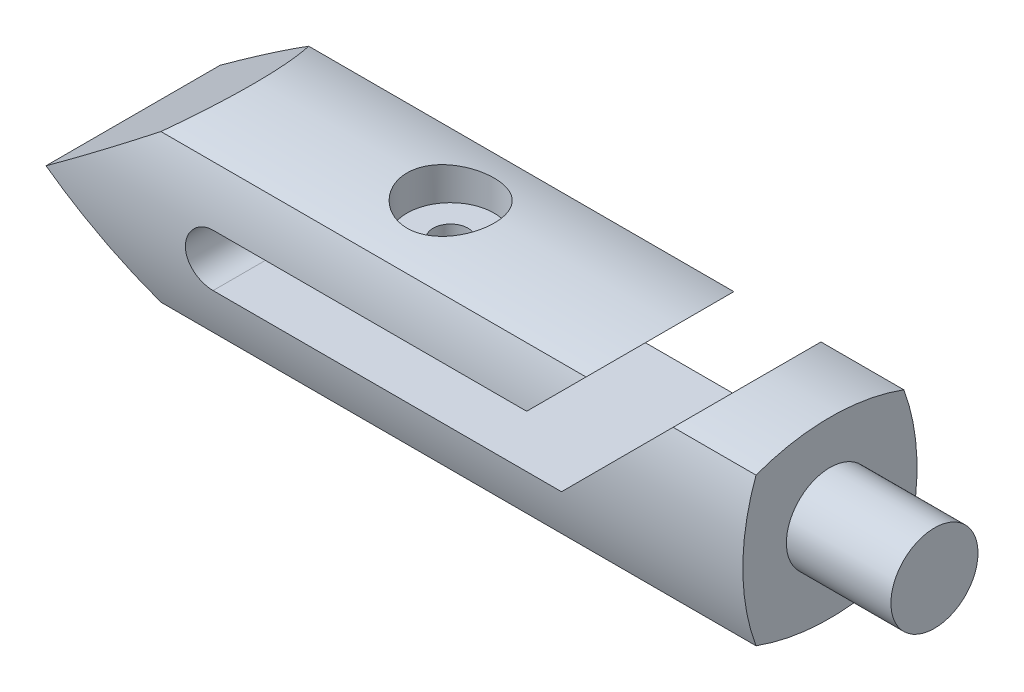
ISO-10303-21;
HEADER;
FILE_DESCRIPTION(('STEP AP214'),'2;1');
FILE_NAME('part.step','',(''),(''),'','','');
FILE_SCHEMA(('AUTOMOTIVE_DESIGN { 1 0 10303 214 1 1 1 1 }'));
ENDSEC;
DATA;
#1=APPLICATION_CONTEXT('core data for automotive mechanical design processes');
#2=APPLICATION_PROTOCOL_DEFINITION('international standard','automotive_design',2000,#1);
#3=PRODUCT_CONTEXT('',#1,'mechanical');
#4=PRODUCT('Part','Part','',(#3));
#5=PRODUCT_RELATED_PRODUCT_CATEGORY('part','',(#4));
#6=PRODUCT_DEFINITION_FORMATION('','',#4);
#7=PRODUCT_DEFINITION_CONTEXT('part definition',#1,'design');
#8=PRODUCT_DEFINITION('design','',#6,#7);
#9=PRODUCT_DEFINITION_SHAPE('','',#8);
#10=(LENGTH_UNIT() NAMED_UNIT(*) SI_UNIT(.MILLI.,.METRE.));
#11=(NAMED_UNIT(*) PLANE_ANGLE_UNIT() SI_UNIT($,.RADIAN.));
#12=(NAMED_UNIT(*) SI_UNIT($,.STERADIAN.) SOLID_ANGLE_UNIT());
#13=UNCERTAINTY_MEASURE_WITH_UNIT(LENGTH_MEASURE(1.E-05),#10,'distance_accuracy_value','');
#14=(GEOMETRIC_REPRESENTATION_CONTEXT(3) GLOBAL_UNCERTAINTY_ASSIGNED_CONTEXT((#13)) GLOBAL_UNIT_ASSIGNED_CONTEXT((#10,
#11,#12)) REPRESENTATION_CONTEXT('',''));
#15=CARTESIAN_POINT('',(0.,0.,0.));
#16=DIRECTION('',(0.,0.,1.));
#17=DIRECTION('',(1.,0.,0.));
#18=AXIS2_PLACEMENT_3D('',#15,#16,#17);
#19=CARTESIAN_POINT('',(80.,-14.5241496511874,0.));
#20=DIRECTION('',(-1.,0.,0.));
#21=DIRECTION('',(0.,0.,1.));
#22=AXIS2_PLACEMENT_3D('',#19,#20,#21);
#23=CYLINDRICAL_SURFACE('',#22,24.5241496511874);
#24=DIRECTION('',(-1.,0.,0.));
#25=VECTOR('',#24,1.);
#26=CARTESIAN_POINT('',(80.,8.48528137423857,-8.48528137423857));
#27=LINE('',#26,#25);
#28=CARTESIAN_POINT('',(80.,8.48528137423857,-8.48528137423857));
#29=VERTEX_POINT('',#28);
#30=CARTESIAN_POINT('',(70.4852813742386,8.48528137423857,-8.48528137423857));
#31=VERTEX_POINT('',#30);
#32=EDGE_CURVE('E248',#29,#31,#27,.T.);
#33=ORIENTED_EDGE('',*,*,#32,.T.);
#34=CARTESIAN_POINT('',(47.4758503488127,-14.5241496511874,0.));
#35=DIRECTION('',(0.707106781186549,-0.707106781186546,0.));
#36=DIRECTION('',(-0.707106781186546,-0.707106781186549,0.));
#37=AXIS2_PLACEMENT_3D('',#34,#35,#36);
#38=ELLIPSE('',#37,34.6823850423765,24.5241496511874);
#39=CARTESIAN_POINT('',(70.4852813742386,8.48528137423856,8.48528137423857));
#40=VERTEX_POINT('',#39);
#41=EDGE_CURVE('E190',#31,#40,#38,.T.);
#42=ORIENTED_EDGE('',*,*,#41,.T.);
#43=DIRECTION('',(-1.,0.,0.));
#44=VECTOR('',#43,1.);
#45=CARTESIAN_POINT('',(80.,8.48528137423856,8.48528137423857));
#46=LINE('',#45,#44);
#47=CARTESIAN_POINT('',(80.,8.48528137423856,8.48528137423857));
#48=VERTEX_POINT('',#47);
#49=EDGE_CURVE('E259',#48,#40,#46,.T.);
#50=ORIENTED_EDGE('',*,*,#49,.F.);
#51=CARTESIAN_POINT('',(80.,-14.5241496511874,0.));
#52=DIRECTION('',(1.,0.,0.));
#53=DIRECTION('',(0.,0.,1.));
#54=AXIS2_PLACEMENT_3D('',#51,#52,#53);
#55=CIRCLE('',#54,24.5241496511874);
#56=EDGE_CURVE('E251',#29,#48,#55,.T.);
#57=ORIENTED_EDGE('',*,*,#56,.F.);
#58=EDGE_LOOP('',(#33,#42,#50,#57));
#59=FACE_BOUND('',#58,.T.);
#60=ADVANCED_FACE('F37',(#59),#23,.T.);
#61=CARTESIAN_POINT('',(80.,14.5241496511874,0.));
#62=DIRECTION('',(-1.,0.,0.));
#63=DIRECTION('',(0.,0.,1.));
#64=AXIS2_PLACEMENT_3D('',#61,#62,#63);
#65=CYLINDRICAL_SURFACE('',#64,24.5241496511874);
#66=CARTESIAN_POINT('',(36.4274618149669,-9.91878279756692,1.99423404330306));
#67=CARTESIAN_POINT('',(36.5396107174262,-9.91878387951594,1.99422914378513));
#68=CARTESIAN_POINT('',(36.6518361731554,-9.91956063360397,1.98477026677701));
#69=CARTESIAN_POINT('',(36.8731828140898,-9.9225835690341,1.94717561648094));
#70=CARTESIAN_POINT('',(36.9823003258081,-9.92483141960828,1.91901862617786));
#71=CARTESIAN_POINT('',(37.1941934107136,-9.93053976466019,1.84484606293275));
#72=CARTESIAN_POINT('',(37.2969724958837,-9.93399958038463,1.79884048443032));
#73=CARTESIAN_POINT('',(37.4933243792085,-9.94174027856262,1.69029359217857));
#74=CARTESIAN_POINT('',(37.5868991571246,-9.94602098386358,1.62775584506402));
#75=CARTESIAN_POINT('',(37.7624342025995,-9.9549314009157,1.48775754496128));
#76=CARTESIAN_POINT('',(37.8443694897502,-9.95956183158808,1.41026571347757));
#77=CARTESIAN_POINT('',(37.9940848321214,-9.96864179702908,1.24262424200629));
#78=CARTESIAN_POINT('',(38.0618642803249,-9.97309132403378,1.15247405949275));
#79=CARTESIAN_POINT('',(38.181422340064,-9.98131288649792,0.961931970770378));
#80=CARTESIAN_POINT('',(38.2331803569177,-9.98508404736901,0.861527101272117));
#81=CARTESIAN_POINT('',(38.3190935872972,-9.99151452425883,0.65341609960103));
#82=CARTESIAN_POINT('',(38.3532491009652,-9.99417385923528,0.545710091956111));
#83=CARTESIAN_POINT('',(38.4029140361771,-9.99807374981551,0.32631236962031));
#84=CARTESIAN_POINT('',(38.4184653849531,-9.99931749535021,0.214630203439155));
#85=CARTESIAN_POINT('',(38.4306113494179,-10.0002546641417,-0.00976557573688327));
#86=CARTESIAN_POINT('',(38.4272062949528,-9.99994811437399,-0.122479170750583));
#87=CARTESIAN_POINT('',(38.4015701990306,-9.99781961597193,-0.34546647047582));
#88=CARTESIAN_POINT('',(38.3793822976169,-9.99600114006806,-0.455745172544806));
#89=CARTESIAN_POINT('',(38.3168786032461,-9.99105507660593,-0.67100838413095));
#90=CARTESIAN_POINT('',(38.2765626316985,-9.98792747615073,-0.775992841479997));
#91=CARTESIAN_POINT('',(38.1788921277876,-9.98070629614845,-0.977841944245001));
#92=CARTESIAN_POINT('',(38.1215156897114,-9.9766114760856,-1.07469594383791));
#93=CARTESIAN_POINT('',(37.9913689733101,-9.96791439848711,-1.25741589796487));
#94=CARTESIAN_POINT('',(37.9185983918504,-9.9633121309599,-1.3432816360696));
#95=CARTESIAN_POINT('',(37.7594737792699,-9.95409985360554,-1.50185153497478));
#96=CARTESIAN_POINT('',(37.6730804520599,-9.94948986078113,-1.57451626919999));
#97=CARTESIAN_POINT('',(37.4892995271567,-9.94079402053666,-1.70431590707003));
#98=CARTESIAN_POINT('',(37.3919119255137,-9.9367081733049,-1.76145080513547));
#99=CARTESIAN_POINT('',(37.1888877575802,-9.92952175902326,-1.85856220639398));
#100=CARTESIAN_POINT('',(37.0832508828721,-9.92642122883369,-1.89853806769411));
#101=CARTESIAN_POINT('',(36.8667332709295,-9.92155756185618,-1.96017326130295));
#102=CARTESIAN_POINT('',(36.7558526431209,-9.91979439717337,-1.98183297565238));
#103=CARTESIAN_POINT('',(36.5323500030333,-9.91780917693866,-2.00616958067166));
#104=CARTESIAN_POINT('',(36.4197341898689,-9.91758252853865,-2.00890304490123));
#105=CARTESIAN_POINT('',(36.1956459444873,-9.91868382758372,-1.99545768529034));
#106=CARTESIAN_POINT('',(36.0841735016966,-9.92001176063949,-1.97927903650156));
#107=CARTESIAN_POINT('',(35.8656968809238,-9.92406876703792,-1.92851561407786));
#108=CARTESIAN_POINT('',(35.7586865961699,-9.92679585261481,-1.8939569502517));
#109=CARTESIAN_POINT('',(35.551982876258,-9.93334291111696,-1.80744148884544));
#110=CARTESIAN_POINT('',(35.4522895561389,-9.93716290122049,-1.75548441779515));
#111=CARTESIAN_POINT('',(35.26279284038,-9.94547740571136,-1.63550560894451));
#112=CARTESIAN_POINT('',(35.1730131914628,-9.94997348127245,-1.56744647508123));
#113=CARTESIAN_POINT('',(35.0061319756589,-9.959129613978,-1.41725031708977));
#114=CARTESIAN_POINT('',(34.9290306267771,-9.96378967394052,-1.33511305093606));
#115=CARTESIAN_POINT('',(34.7894999262584,-9.97276407920029,-1.15884676404799));
#116=CARTESIAN_POINT('',(34.7271076192201,-9.97707753395946,-1.06468836749474));
#117=CARTESIAN_POINT('',(34.6190195674161,-9.9848616206904,-0.867199529201713));
#118=CARTESIAN_POINT('',(34.5733236688444,-9.98833226042602,-0.763869171964319));
#119=CARTESIAN_POINT('',(34.4999846709961,-9.99403787574732,-0.551090485409505));
#120=CARTESIAN_POINT('',(34.4723205998467,-9.99627428633419,-0.441649424615883));
#121=CARTESIAN_POINT('',(34.4357636338553,-9.99926739888673,-0.219656585902366));
#122=CARTESIAN_POINT('',(34.426870394789,-10.0000241279872,-0.10710486506488));
#123=CARTESIAN_POINT('',(34.4281125479617,-9.99997475904181,0.117558752308689));
#124=CARTESIAN_POINT('',(34.4381917133107,-9.99917327869674,0.229670964829407));
#125=CARTESIAN_POINT('',(34.4769765751515,-9.99610895300196,0.450604543013426));
#126=CARTESIAN_POINT('',(34.5056822851811,-9.99384610659015,0.559425906284876));
#127=CARTESIAN_POINT('',(34.5808878132343,-9.98811548672665,0.770679710877488));
#128=CARTESIAN_POINT('',(34.6273847023371,-9.98464791161532,0.873113200593169));
#129=CARTESIAN_POINT('',(34.7368466796898,-9.97689787677331,1.0687283584638));
#130=CARTESIAN_POINT('',(34.7998114837321,-9.97261543110623,1.16191018624808));
#131=CARTESIAN_POINT('',(34.9406238598056,-9.96370373201027,1.3366530766732));
#132=CARTESIAN_POINT('',(35.0185112405738,-9.95907357154377,1.41818201368821));
#133=CARTESIAN_POINT('',(35.1868874368628,-9.94999734378366,1.56704257270282));
#134=CARTESIAN_POINT('',(35.277379304508,-9.94555132141762,1.63437074608838));
#135=CARTESIAN_POINT('',(35.4685683054161,-9.93733902638497,1.75300935209794));
#136=CARTESIAN_POINT('',(35.5692840696393,-9.93357403076966,1.8042898210522));
#137=CARTESIAN_POINT('',(35.7778571652447,-9.92716649272995,1.8891486623785));
#138=CARTESIAN_POINT('',(35.8857061163373,-9.92452265928407,1.92274740611571));
#139=CARTESIAN_POINT('',(36.0664045825854,-9.92133837222752,1.96271812167535));
#140=CARTESIAN_POINT('',(36.1380918860322,-9.92038443324707,1.97452093798435));
#141=CARTESIAN_POINT('',(36.2823293776411,-9.9191062965746,1.99028047462704));
#142=CARTESIAN_POINT('',(36.3548795636816,-9.91878209733451,1.99423721424842));
#143=CARTESIAN_POINT('',(36.4274618149669,-9.91878279756692,1.99423404330306));
#144=B_SPLINE_CURVE_WITH_KNOTS('',3,(#66,#67,#68,#69,#70,#71,#72,#73,#74,#75,#76,#77,#78,#79,
#80,#81,#82,#83,#84,#85,#86,#87,#88,#89,#90,#91,#92,#93,#94,#95,#96,#97,#98,#99,#100,#101,#102,
#103,#104,#105,#106,#107,#108,#109,#110,#111,#112,#113,#114,#115,#116,#117,#118,#119,#120,#121,
#122,#123,#124,#125,#126,#127,#128,#129,#130,#131,#132,#133,#134,#135,#136,#137,#138,#139,#140,
#141,#142,#143),.UNSPECIFIED.,.T.,.F.,(4,2,2,2,2,2,2,2,2,2,2,2,2,2,2,2,2,2,2,2,2,2,2,2,2,2,2,2,
2,2,2,2,2,2,2,2,2,2,4),(0.,0.336181721876391,0.672745567258664,1.00912122278101,
1.34542436807037,1.68243871436159,2.01946750920759,2.35692775427698,2.69438224508603,
3.03107479102768,3.36776147845564,3.70367696258342,4.03959575608857,4.37594774715791,
4.71230636213535,5.0496536092943,5.38700097765134,5.72436096455003,6.06171391457386,
6.39805802616283,6.73439902455492,7.07026350349091,7.40613326183175,7.74279084986612,
8.07945422616162,8.41695663863483,8.75445594198052,9.09156201385299,9.42866190373632,
9.76476433216564,10.1008670048747,10.4369143695644,10.7729559350427,11.109906760192,
11.4469393188911,11.784597468342,12.1218657406696,12.3394415319915,12.5570167884555),.UNSPECIFIED.);
#145=CARTESIAN_POINT('',(36.4274618149669,-9.91878279756692,1.99423404330306));
#146=VERTEX_POINT('',#145);
#147=EDGE_CURVE('E44',#146,#146,#144,.T.);
#148=ORIENTED_EDGE('',*,*,#147,.T.);
#149=EDGE_LOOP('',(#148));
#150=FACE_BOUND('',#149,.T.);
#151=CARTESIAN_POINT('',(-19.9907769901119,14.5241496511874,0.));
#152=DIRECTION('',(-0.587785252292474,-0.809016994374947,0.));
#153=DIRECTION('',(-0.809016994374947,0.587785252292474,0.));
#154=AXIS2_PLACEMENT_3D('',#151,#152,#153);
#155=ELLIPSE('',#154,41.7229754498578,24.5241496511874);
#156=CARTESIAN_POINT('',(11.6789878736127,-8.48528137423857,-8.48528137423857));
#157=VERTEX_POINT('',#156);
#158=CARTESIAN_POINT('',(11.6789878736127,-8.48528137423857,8.48528137423857));
#159=VERTEX_POINT('',#158);
#160=EDGE_CURVE('E289',#157,#159,#155,.T.);
#161=ORIENTED_EDGE('',*,*,#160,.F.);
#162=DIRECTION('',(-1.,0.,0.));
#163=VECTOR('',#162,1.);
#164=CARTESIAN_POINT('',(80.,-8.48528137423857,-8.48528137423857));
#165=LINE('',#164,#163);
#166=CARTESIAN_POINT('',(80.,-8.48528137423857,-8.48528137423857));
#167=VERTEX_POINT('',#166);
#168=EDGE_CURVE('E255',#167,#157,#165,.T.);
#169=ORIENTED_EDGE('',*,*,#168,.F.);
#170=CARTESIAN_POINT('',(80.,14.5241496511874,0.));
#171=DIRECTION('',(1.,0.,0.));
#172=DIRECTION('',(0.,0.,-1.));
#173=AXIS2_PLACEMENT_3D('',#170,#171,#172);
#174=CIRCLE('',#173,24.5241496511874);
#175=CARTESIAN_POINT('',(80.,-8.48528137423857,8.48528137423857));
#176=VERTEX_POINT('',#175);
#177=EDGE_CURVE('E303',#176,#167,#174,.T.);
#178=ORIENTED_EDGE('',*,*,#177,.F.);
#179=DIRECTION('',(-1.,0.,0.));
#180=VECTOR('',#179,1.);
#181=CARTESIAN_POINT('',(80.,-8.48528137423857,8.48528137423857));
#182=LINE('',#181,#180);
#183=EDGE_CURVE('E310',#176,#159,#182,.T.);
#184=ORIENTED_EDGE('',*,*,#183,.T.);
#185=EDGE_LOOP('',(#161,#169,#178,#184));
#186=FACE_BOUND('',#185,.T.);
#187=ADVANCED_FACE('F45',(#150,#186),#65,.T.);
#188=CARTESIAN_POINT('',(80.,0.,14.5241496511873));
#189=DIRECTION('',(-1.,0.,0.));
#190=DIRECTION('',(0.,0.,1.));
#191=AXIS2_PLACEMENT_3D('',#188,#189,#190);
#192=CYLINDRICAL_SURFACE('',#191,24.5241496511874);
#193=DIRECTION('',(-1.,0.,0.));
#194=VECTOR('',#193,1.);
#195=CARTESIAN_POINT('',(80.,3.,-9.81581575786434));
#196=LINE('',#195,#194);
#197=CARTESIAN_POINT('',(55.,3.,-9.81581575786434));
#198=VERTEX_POINT('',#197);
#199=CARTESIAN_POINT('',(19.,3.,-9.81581575786434));
#200=VERTEX_POINT('',#199);
#201=EDGE_CURVE('E134',#198,#200,#196,.T.);
#202=ORIENTED_EDGE('',*,*,#201,.T.);
#203=CARTESIAN_POINT('',(19.,3.,-9.81581575786434));
#204=CARTESIAN_POINT('',(18.9159581160124,3.00000845084196,-9.81581145497862));
#205=CARTESIAN_POINT('',(18.8319204963024,2.99646853759129,-9.81625094060136));
#206=CARTESIAN_POINT('',(18.664452727367,2.98235744015164,-9.81798568516386));
#207=CARTESIAN_POINT('',(18.5810225326003,2.97178678869135,-9.81928087926537));
#208=CARTESIAN_POINT('',(18.4154392675195,2.94369384169545,-9.82269352253626));
#209=CARTESIAN_POINT('',(18.3332849928944,2.92617857509987,-9.82481014026211));
#210=CARTESIAN_POINT('',(18.1707754863183,2.88434334207964,-9.82980114295365));
#211=CARTESIAN_POINT('',(18.0904202431902,2.86002341794395,-9.83267552321006));
#212=CARTESIAN_POINT('',(17.8528488125263,2.77707037687542,-9.8423220854026));
#213=CARTESIAN_POINT('',(17.6990342186838,2.7084281645373,-9.85011973385544));
#214=CARTESIAN_POINT('',(17.405204709813,2.54652833477299,-9.86756395041019));
#215=CARTESIAN_POINT('',(17.2651886506251,2.45327276062299,-9.87721036501874));
#216=CARTESIAN_POINT('',(17.0020707993755,2.24424237310175,-9.8973232696192));
#217=CARTESIAN_POINT('',(16.879051473348,2.1283639265146,-9.90779339591513));
#218=CARTESIAN_POINT('',(16.6541477560292,1.87759299766197,-9.9283421820244));
#219=CARTESIAN_POINT('',(16.5522665856149,1.74269762298811,-9.93842078198995));
#220=CARTESIAN_POINT('',(16.3722404196189,1.45720411210512,-9.95708742327201));
#221=CARTESIAN_POINT('',(16.2941710108273,1.30655796834562,-9.96567068163192));
#222=CARTESIAN_POINT('',(16.1644749648453,0.994180082275956,-9.98033855169631));
#223=CARTESIAN_POINT('',(16.1128458186752,0.832449393456734,-9.98642340046998));
#224=CARTESIAN_POINT('',(16.0377389031857,0.50334311382209,-9.99538359571057));
#225=CARTESIAN_POINT('',(16.0141216504363,0.335999795323433,-9.99827483953598));
#226=CARTESIAN_POINT('',(15.9952767735246,-0.00030237620532862,-10.000576353286));
#227=CARTESIAN_POINT('',(16.0000487651077,-0.169261207338216,-9.99998667032566));
#228=CARTESIAN_POINT('',(16.0377359374063,-0.503040463753467,-9.99540552373128));
#229=CARTESIAN_POINT('',(16.0705003118933,-0.667878202042692,-9.99143228902271));
#230=CARTESIAN_POINT('',(16.1630064088251,-0.989696912406668,-9.98055103935256));
#231=CARTESIAN_POINT('',(16.2227484803348,-1.14667778279207,-9.97364298641737));
#232=CARTESIAN_POINT('',(16.3676762914144,-1.44879829042551,-9.95763681003417));
#233=CARTESIAN_POINT('',(16.4529279570903,-1.5939059904158,-9.94853302397992));
#234=CARTESIAN_POINT('',(16.6464034985944,-1.8678056987294,-9.92915480375318));
#235=CARTESIAN_POINT('',(16.754627407048,-1.99659768388062,-9.91888036791812));
#236=CARTESIAN_POINT('',(16.9918032180423,-2.23508622992994,-9.89823260363041));
#237=CARTESIAN_POINT('',(17.1208837176772,-2.34465490705928,-9.88785906373503));
#238=CARTESIAN_POINT('',(17.3957198663395,-2.54062393929399,-9.8682442536347));
#239=CARTESIAN_POINT('',(17.5414804662569,-2.6270173900858,-9.85900332129808));
#240=CARTESIAN_POINT('',(17.8456708868832,-2.77418821752534,-9.84269883775925));
#241=CARTESIAN_POINT('',(18.0041130087376,-2.83494035477096,-9.83563743375076));
#242=CARTESIAN_POINT('',(18.3289404402981,-2.92885088166213,-9.8245263367096));
#243=CARTESIAN_POINT('',(18.4953133802896,-2.96205084568168,-9.82047210703893));
#244=CARTESIAN_POINT('',(18.7190664113999,-2.98735135547406,-9.81737175815089));
#245=CARTESIAN_POINT('',(18.7751965189995,-2.99209685986428,-9.8167886672682));
#246=CARTESIAN_POINT('',(18.8875431742416,-2.99841693498194,-9.81601112392274));
#247=CARTESIAN_POINT('',(18.9437594184302,-2.99999681734021,-9.81581602045592));
#248=CARTESIAN_POINT('',(19.,-3.,-9.81581575786435));
#249=B_SPLINE_CURVE_WITH_KNOTS('',3,(#203,#204,#205,#206,#207,#208,#209,#210,#211,#212,#213,
#214,#215,#216,#217,#218,#219,#220,#221,#222,#223,#224,#225,#226,#227,#228,#229,#230,#231,#232,
#233,#234,#235,#236,#237,#238,#239,#240,#241,#242,#243,#244,#245,#246,#247,#248),.UNSPECIFIED.,
.F.,.F.,(4,2,2,2,2,2,2,2,2,2,2,2,2,2,2,2,2,2,2,2,2,2,4),(0.,0.25204239169317,0.504065687963076,
0.755834549262021,1.00760184592548,1.5108577868495,2.01407196315652,2.51964782380479,
3.02530066390625,3.53254230549588,4.03973580479146,4.54439301955133,5.04904340368218,
5.5509920542682,6.05294719976308,6.55621095225397,7.05947541948773,7.56597042749188,
8.07261616223859,8.57975944482824,9.08613608375071,9.25507037230103,9.42372096604725),.UNSPECIFIED.);
#250=CARTESIAN_POINT('',(19.,-3.,-9.81581575786434));
#251=VERTEX_POINT('',#250);
#252=EDGE_CURVE('E138',#200,#251,#249,.T.);
#253=ORIENTED_EDGE('',*,*,#252,.T.);
#254=DIRECTION('',(-1.,0.,0.));
#255=VECTOR('',#254,1.);
#256=CARTESIAN_POINT('',(80.,-3.,-9.81581575786434));
#257=LINE('',#256,#255);
#258=CARTESIAN_POINT('',(59.,-3.,-9.81581575786434));
#259=VERTEX_POINT('',#258);
#260=EDGE_CURVE('E163',#251,#259,#257,.F.);
#261=ORIENTED_EDGE('',*,*,#260,.T.);
#262=CARTESIAN_POINT('',(62.,0.,14.5241496511873));
#263=DIRECTION('',(0.707106781186549,-0.707106781186546,0.));
#264=DIRECTION('',(-0.707106781186546,-0.707106781186549,0.));
#265=AXIS2_PLACEMENT_3D('',#262,#263,#264);
#266=ELLIPSE('',#265,34.6823850423765,24.5241496511874);
#267=EDGE_CURVE('E140',#259,#31,#266,.T.);
#268=ORIENTED_EDGE('',*,*,#267,.T.);
#269=ORIENTED_EDGE('',*,*,#32,.F.);
#270=CARTESIAN_POINT('',(80.,0.,14.5241496511873));
#271=DIRECTION('',(1.,0.,0.));
#272=DIRECTION('',(0.,0.,-1.));
#273=AXIS2_PLACEMENT_3D('',#270,#271,#272);
#274=CIRCLE('',#273,24.5241496511874);
#275=EDGE_CURVE('E308',#167,#29,#274,.T.);
#276=ORIENTED_EDGE('',*,*,#275,.F.);
#277=ORIENTED_EDGE('',*,*,#168,.T.);
#278=CARTESIAN_POINT('',(0.,0.,14.5241496511873));
#279=DIRECTION('',(-0.587785252292474,-0.809016994374947,0.));
#280=DIRECTION('',(-0.809016994374947,0.587785252292474,0.));
#281=AXIS2_PLACEMENT_3D('',#278,#279,#280);
#282=ELLIPSE('',#281,41.7229754498578,24.5241496511874);
#283=CARTESIAN_POINT('',(0.,0.,-10.));
#284=VERTEX_POINT('',#283);
#285=EDGE_CURVE('E295',#284,#157,#282,.T.);
#286=ORIENTED_EDGE('',*,*,#285,.F.);
#287=CARTESIAN_POINT('',(0.,0.,14.5241496511873));
#288=DIRECTION('',(0.587785252292474,-0.809016994374947,0.));
#289=DIRECTION('',(-0.809016994374947,-0.587785252292474,0.));
#290=AXIS2_PLACEMENT_3D('',#287,#288,#289);
#291=ELLIPSE('',#290,41.7229754498578,24.5241496511874);
#292=CARTESIAN_POINT('',(11.6789878736127,8.48528137423857,-8.48528137423857));
#293=VERTEX_POINT('',#292);
#294=EDGE_CURVE('E302',#284,#293,#291,.T.);
#295=ORIENTED_EDGE('',*,*,#294,.T.);
#296=CARTESIAN_POINT('',(60.4852813742386,8.48528137423857,-8.48528137423857));
#297=VERTEX_POINT('',#296);
#298=EDGE_CURVE('E147',#297,#293,#27,.T.);
#299=ORIENTED_EDGE('',*,*,#298,.F.);
#300=CARTESIAN_POINT('',(52.,0.,14.5241496511873));
#301=DIRECTION('',(-0.707106781186549,0.707106781186546,0.));
#302=DIRECTION('',(-0.707106781186546,-0.707106781186549,0.));
#303=AXIS2_PLACEMENT_3D('',#300,#301,#302);
#304=ELLIPSE('',#303,34.6823850423765,24.5241496511874);
#305=EDGE_CURVE('E63',#297,#198,#304,.T.);
#306=ORIENTED_EDGE('',*,*,#305,.T.);
#307=EDGE_LOOP('',(#202,#253,#261,#268,#269,#276,#277,#286,#295,#299,#306));
#308=FACE_BOUND('',#307,.T.);
#309=ADVANCED_FACE('F146',(#308),#192,.T.);
#310=CARTESIAN_POINT('',(80.,0.,-14.5241496511873));
#311=DIRECTION('',(-1.,0.,0.));
#312=DIRECTION('',(0.,0.,1.));
#313=AXIS2_PLACEMENT_3D('',#310,#311,#312);
#314=CYLINDRICAL_SURFACE('',#313,24.5241496511874);
#315=ORIENTED_EDGE('',*,*,#49,.T.);
#316=CARTESIAN_POINT('',(62.,0.,-14.5241496511873));
#317=DIRECTION('',(0.707106781186549,-0.707106781186546,0.));
#318=DIRECTION('',(-0.707106781186546,-0.707106781186549,0.));
#319=AXIS2_PLACEMENT_3D('',#316,#317,#318);
#320=ELLIPSE('',#319,34.6823850423765,24.5241496511874);
#321=CARTESIAN_POINT('',(59.,-3.,9.81581575786434));
#322=VERTEX_POINT('',#321);
#323=EDGE_CURVE('E151',#40,#322,#320,.T.);
#324=ORIENTED_EDGE('',*,*,#323,.T.);
#325=DIRECTION('',(-1.,0.,0.));
#326=VECTOR('',#325,1.);
#327=CARTESIAN_POINT('',(80.,-3.,9.81581575786434));
#328=LINE('',#327,#326);
#329=CARTESIAN_POINT('',(19.,-3.,9.81581575786434));
#330=VERTEX_POINT('',#329);
#331=EDGE_CURVE('E210',#322,#330,#328,.T.);
#332=ORIENTED_EDGE('',*,*,#331,.T.);
#333=CARTESIAN_POINT('',(19.,-3.,9.81581575786434));
#334=CARTESIAN_POINT('',(18.9159581160124,-3.00000845084196,9.81581145497862));
#335=CARTESIAN_POINT('',(18.8319204963024,-2.9964685375913,9.81625094060136));
#336=CARTESIAN_POINT('',(18.664452727367,-2.98235744015164,9.81798568516386));
#337=CARTESIAN_POINT('',(18.5810225326003,-2.97178678869136,9.81928087926537));
#338=CARTESIAN_POINT('',(18.4154392675195,-2.94369384169545,9.82269352253626));
#339=CARTESIAN_POINT('',(18.3332849928944,-2.92617857509987,9.82481014026211));
#340=CARTESIAN_POINT('',(18.1707754863183,-2.88434334207964,9.82980114295365));
#341=CARTESIAN_POINT('',(18.0904202431902,-2.86002341794395,9.83267552321006));
#342=CARTESIAN_POINT('',(17.8528488125263,-2.77707037687543,9.8423220854026));
#343=CARTESIAN_POINT('',(17.6990342186838,-2.7084281645373,9.85011973385544));
#344=CARTESIAN_POINT('',(17.405204709813,-2.546528334773,9.86756395041019));
#345=CARTESIAN_POINT('',(17.2651886506251,-2.45327276062299,9.87721036501874));
#346=CARTESIAN_POINT('',(17.0020707993755,-2.24424237310176,9.8973232696192));
#347=CARTESIAN_POINT('',(16.879051473348,-2.1283639265146,9.90779339591513));
#348=CARTESIAN_POINT('',(16.6541477560292,-1.87759299766197,9.92834218202439));
#349=CARTESIAN_POINT('',(16.5522665856149,-1.74269762298811,9.93842078198994));
#350=CARTESIAN_POINT('',(16.3722404196189,-1.45720411210512,9.957087423272));
#351=CARTESIAN_POINT('',(16.2941710108273,-1.30655796834562,9.96567068163192));
#352=CARTESIAN_POINT('',(16.1644749648453,-0.99418008227596,9.98033855169631));
#353=CARTESIAN_POINT('',(16.1128458186752,-0.832449393456739,9.98642340046998));
#354=CARTESIAN_POINT('',(16.0377389031857,-0.503343113822096,9.99538359571057));
#355=CARTESIAN_POINT('',(16.0141216504363,-0.335999795323438,9.99827483953598));
#356=CARTESIAN_POINT('',(15.9952767735246,0.000302376205323876,10.000576353286));
#357=CARTESIAN_POINT('',(16.0000487651077,0.169261207338211,9.99998667032566));
#358=CARTESIAN_POINT('',(16.0377359374063,0.503040463753463,9.99540552373128));
#359=CARTESIAN_POINT('',(16.0705003118933,0.667878202042688,9.99143228902271));
#360=CARTESIAN_POINT('',(16.1630064088251,0.989696912406665,9.98055103935255));
#361=CARTESIAN_POINT('',(16.2227484803348,1.14667778279206,9.97364298641737));
#362=CARTESIAN_POINT('',(16.3676762914144,1.44879829042551,9.95763681003416));
#363=CARTESIAN_POINT('',(16.4529279570903,1.5939059904158,9.94853302397992));
#364=CARTESIAN_POINT('',(16.6464034985944,1.8678056987294,9.92915480375318));
#365=CARTESIAN_POINT('',(16.754627407048,1.99659768388062,9.91888036791812));
#366=CARTESIAN_POINT('',(16.9918032180423,2.23508622992993,9.89823260363041));
#367=CARTESIAN_POINT('',(17.1208837176772,2.34465490705927,9.88785906373503));
#368=CARTESIAN_POINT('',(17.3957198663395,2.54062393929398,9.8682442536347));
#369=CARTESIAN_POINT('',(17.5414804662569,2.6270173900858,9.85900332129807));
#370=CARTESIAN_POINT('',(17.8456708868832,2.77418821752534,9.84269883775925));
#371=CARTESIAN_POINT('',(18.0041130087376,2.83494035477096,9.83563743375076));
#372=CARTESIAN_POINT('',(18.3289404402981,2.92885088166212,9.8245263367096));
#373=CARTESIAN_POINT('',(18.4953133802896,2.96205084568167,9.82047210703895));
#374=CARTESIAN_POINT('',(18.7190664113999,2.98735135547405,9.8173717581509));
#375=CARTESIAN_POINT('',(18.7751965189995,2.99209685986428,9.8167886672682));
#376=CARTESIAN_POINT('',(18.8875431742416,2.99841693498194,9.81601112392274));
#377=CARTESIAN_POINT('',(18.9437594184302,2.99999681734021,9.81581602045591));
#378=CARTESIAN_POINT('',(19.,3.,9.81581575786434));
#379=B_SPLINE_CURVE_WITH_KNOTS('',3,(#333,#334,#335,#336,#337,#338,#339,#340,#341,#342,#343,
#344,#345,#346,#347,#348,#349,#350,#351,#352,#353,#354,#355,#356,#357,#358,#359,#360,#361,#362,
#363,#364,#365,#366,#367,#368,#369,#370,#371,#372,#373,#374,#375,#376,#377,#378),.UNSPECIFIED.,
.F.,.F.,(4,2,2,2,2,2,2,2,2,2,2,2,2,2,2,2,2,2,2,2,2,2,4),(0.,0.25204239169317,0.504065687963072,
0.755834549262018,1.00760184592548,1.5108577868495,2.01407196315652,2.51964782380479,
3.02530066390625,3.53254230549588,4.03973580479146,4.54439301955132,5.04904340368218,
5.5509920542682,6.05294719976308,6.55621095225397,7.05947541948773,7.56597042749188,
8.07261616223859,8.57975944482824,9.08613608375071,9.25507037230103,9.42372096604725),.UNSPECIFIED.);
#380=CARTESIAN_POINT('',(19.,3.,9.81581575786434));
#381=VERTEX_POINT('',#380);
#382=EDGE_CURVE('E178',#330,#381,#379,.T.);
#383=ORIENTED_EDGE('',*,*,#382,.T.);
#384=DIRECTION('',(-1.,0.,0.));
#385=VECTOR('',#384,1.);
#386=CARTESIAN_POINT('',(80.,3.,9.81581575786434));
#387=LINE('',#386,#385);
#388=CARTESIAN_POINT('',(55.,3.,9.81581575786434));
#389=VERTEX_POINT('',#388);
#390=EDGE_CURVE('E187',#381,#389,#387,.F.);
#391=ORIENTED_EDGE('',*,*,#390,.T.);
#392=CARTESIAN_POINT('',(52.,0.,-14.5241496511873));
#393=DIRECTION('',(-0.707106781186549,0.707106781186546,0.));
#394=DIRECTION('',(-0.707106781186546,-0.707106781186549,0.));
#395=AXIS2_PLACEMENT_3D('',#392,#393,#394);
#396=ELLIPSE('',#395,34.6823850423765,24.5241496511874);
#397=CARTESIAN_POINT('',(60.4852813742386,8.48528137423856,8.48528137423857));
#398=VERTEX_POINT('',#397);
#399=EDGE_CURVE('E145',#389,#398,#396,.T.);
#400=ORIENTED_EDGE('',*,*,#399,.T.);
#401=CARTESIAN_POINT('',(11.6789878736127,8.48528137423856,8.48528137423857));
#402=VERTEX_POINT('',#401);
#403=EDGE_CURVE('E266',#398,#402,#46,.T.);
#404=ORIENTED_EDGE('',*,*,#403,.T.);
#405=CARTESIAN_POINT('',(0.,0.,-14.5241496511873));
#406=DIRECTION('',(0.587785252292474,-0.809016994374947,0.));
#407=DIRECTION('',(-0.809016994374947,-0.587785252292474,0.));
#408=AXIS2_PLACEMENT_3D('',#405,#406,#407);
#409=ELLIPSE('',#408,41.7229754498578,24.5241496511874);
#410=CARTESIAN_POINT('',(0.,0.,10.));
#411=VERTEX_POINT('',#410);
#412=EDGE_CURVE('E297',#402,#411,#409,.T.);
#413=ORIENTED_EDGE('',*,*,#412,.T.);
#414=CARTESIAN_POINT('',(0.,0.,-14.5241496511873));
#415=DIRECTION('',(-0.587785252292474,-0.809016994374947,0.));
#416=DIRECTION('',(-0.809016994374947,0.587785252292474,0.));
#417=AXIS2_PLACEMENT_3D('',#414,#415,#416);
#418=ELLIPSE('',#417,41.7229754498578,24.5241496511874);
#419=EDGE_CURVE('E287',#159,#411,#418,.T.);
#420=ORIENTED_EDGE('',*,*,#419,.F.);
#421=ORIENTED_EDGE('',*,*,#183,.F.);
#422=CARTESIAN_POINT('',(80.,0.,-14.5241496511873));
#423=DIRECTION('',(1.,0.,0.));
#424=DIRECTION('',(0.,0.,1.));
#425=AXIS2_PLACEMENT_3D('',#422,#423,#424);
#426=CIRCLE('',#425,24.5241496511874);
#427=EDGE_CURVE('E68',#48,#176,#426,.T.);
#428=ORIENTED_EDGE('',*,*,#427,.F.);
#429=EDGE_LOOP('',(#315,#324,#332,#383,#391,#400,#404,#413,#420,#421,#428));
#430=FACE_BOUND('',#429,.T.);
#431=ADVANCED_FACE('F192',(#430),#314,.T.);
#432=CARTESIAN_POINT('',(36.4274618149669,9.49113147685785,4.96992841545921));
#433=CARTESIAN_POINT('',(36.2885654697479,9.49112989054858,4.96993128320022));
#434=CARTESIAN_POINT('',(36.1497045457016,9.49233175950607,4.96413777976222));
#435=CARTESIAN_POINT('',(35.8729430572493,9.49709993331018,4.94101569183181));
#436=CARTESIAN_POINT('',(35.7350426755279,9.50066667615679,4.92368497052069));
#437=CARTESIAN_POINT('',(35.4611754098703,9.51006286149759,4.8776114439388));
#438=CARTESIAN_POINT('',(35.3252095220988,9.51589342893134,4.84886296479369));
#439=CARTESIAN_POINT('',(35.0561906627736,9.52964659781938,4.78017037412584));
#440=CARTESIAN_POINT('',(34.9231387834459,9.53756996964124,4.74022213960614));
#441=CARTESIAN_POINT('',(34.6611142553664,9.55526333994881,4.64950710587216));
#442=CARTESIAN_POINT('',(34.5321361498255,9.56503073427539,4.59875555055219));
#443=CARTESIAN_POINT('',(34.2788971746808,9.58614169647089,4.48675979555837));
#444=CARTESIAN_POINT('',(34.1546380661447,9.59748584554573,4.42551172482624));
#445=CARTESIAN_POINT('',(33.911773447445,9.62141975359037,4.29300853177652));
#446=CARTESIAN_POINT('',(33.7931654908028,9.63400896615612,4.22175779348495));
#447=CARTESIAN_POINT('',(33.5622843761664,9.66008914031604,4.06970029426311));
#448=CARTESIAN_POINT('',(33.4500136080163,9.67358043796449,3.98888996337153));
#449=CARTESIAN_POINT('',(33.2311939271179,9.70126324216399,3.81719031473778));
#450=CARTESIAN_POINT('',(33.1247368174313,9.71546150793852,3.72618506863727));
#451=CARTESIAN_POINT('',(32.9197990263605,9.74400076387225,3.53554554589436));
#452=CARTESIAN_POINT('',(32.8213213162226,9.75834180498425,3.4359080832362));
#453=CARTESIAN_POINT('',(32.6330788992067,9.78675565672325,3.22873409926689));
#454=CARTESIAN_POINT('',(32.5433116390531,9.80082854497538,3.12119990904253));
#455=CARTESIAN_POINT('',(32.3730436373464,9.82832251111225,2.89889070980467));
#456=CARTESIAN_POINT('',(32.2925463226141,9.84174334689964,2.78411304721399));
#457=CARTESIAN_POINT('',(32.1407601115214,9.867664904524,2.54707999722412));
#458=CARTESIAN_POINT('',(32.0695577310381,9.88015657185519,2.42476808123477));
#459=CARTESIAN_POINT('',(31.9377067996527,9.90373607021439,2.17443776311286));
#460=CARTESIAN_POINT('',(31.8770622097406,9.91482337394095,2.04641724179935));
#461=CARTESIAN_POINT('',(31.7117714180197,9.94546739018998,1.65522909762556));
#462=CARTESIAN_POINT('',(31.6235845242409,9.96243877560154,1.38464778418398));
#463=CARTESIAN_POINT('',(31.49519566268,9.98726635779405,0.835991125718323));
#464=CARTESIAN_POINT('',(31.4543539150509,9.99524404573315,0.558068887110443));
#465=CARTESIAN_POINT('',(31.4197253003256,10.0015904081913,-0.00082630053980853));
#466=CARTESIAN_POINT('',(31.4259337288232,9.99996004339429,-0.281798941776387));
#467=CARTESIAN_POINT('',(31.4847715884482,9.98733815292176,-0.834380859114126));
#468=CARTESIAN_POINT('',(31.5367128195851,9.9764854910317,-1.10606716448385));
#469=CARTESIAN_POINT('',(31.6844426599756,9.9467627518072,-1.63677725226291));
#470=CARTESIAN_POINT('',(31.7802330716264,9.92789234490989,-1.89580051368007));
#471=CARTESIAN_POINT('',(32.013575566052,9.8839964595344,-2.39578266258806));
#472=CARTESIAN_POINT('',(32.1513954806712,9.85893170791922,-2.63661296141762));
#473=CARTESIAN_POINT('',(32.4646858291906,9.80538451267041,-3.09197791286804));
#474=CARTESIAN_POINT('',(32.6401607565166,9.77690166132908,-3.30650942241241));
#475=CARTESIAN_POINT('',(33.0275494826198,9.71903160719063,-3.70727446832944));
#476=CARTESIAN_POINT('',(33.2400655295425,9.68963736770865,-3.89292529866188));
#477=CARTESIAN_POINT('',(33.6935170598738,9.63372699795079,-4.22605360800891));
#478=CARTESIAN_POINT('',(33.9344531236193,9.60721092646838,-4.37353030731089));
#479=CARTESIAN_POINT('',(34.4387632237934,9.56002682373061,-4.62633922793106));
#480=CARTESIAN_POINT('',(34.7021874658419,9.53937234764845,-4.73157399208178));
#481=CARTESIAN_POINT('',(35.2434990428136,9.50643448816495,-4.89612663673533));
#482=CARTESIAN_POINT('',(35.5213844065209,9.49414996704365,-4.95545075797687));
#483=CARTESIAN_POINT('',(36.0784402268979,9.47956490797415,-5.02562226516219));
#484=CARTESIAN_POINT('',(36.3575001126488,9.47709084561209,-5.03731229219958));
#485=CARTESIAN_POINT('',(36.9135827157729,9.48193933580449,-5.01415428191593));
#486=CARTESIAN_POINT('',(37.1906055525221,9.48926130961113,-4.97930899389207));
#487=CARTESIAN_POINT('',(37.7318970712818,9.51271785257822,-4.86479611700705));
#488=CARTESIAN_POINT('',(37.9962657983847,9.52876330767241,-4.78558153593979));
#489=CARTESIAN_POINT('',(38.5079755645804,9.56778855832293,-4.58506254629861));
#490=CARTESIAN_POINT('',(38.7553151522587,9.59076894405554,-4.46375455536067));
#491=CARTESIAN_POINT('',(39.2296255994549,9.64147569600854,-4.18059288924195));
#492=CARTESIAN_POINT('',(39.4562760966734,9.66926199158361,-4.0182135329568));
#493=CARTESIAN_POINT('',(39.8794135707974,9.72630463752091,-3.65821259382352));
#494=CARTESIAN_POINT('',(40.075897311385,9.75556114516261,-3.46058723466054));
#495=CARTESIAN_POINT('',(40.4363349456981,9.81283502622682,-3.03191573193543));
#496=CARTESIAN_POINT('',(40.5997179946981,9.84082508006214,-2.80038540090991));
#497=CARTESIAN_POINT('',(40.8852596449504,9.89194231430196,-2.31265639582262));
#498=CARTESIAN_POINT('',(41.0074200201479,9.9150697039465,-2.05645878388378));
#499=CARTESIAN_POINT('',(41.2062281581127,9.95376420913303,-1.52819528853983));
#500=CARTESIAN_POINT('',(41.283140572581,9.96937518801117,-1.2562321089551));
#501=CARTESIAN_POINT('',(41.3900903512288,9.99148908935866,-0.702734388449571));
#502=CARTESIAN_POINT('',(41.4201335933613,9.99799315393316,-0.421201052266283));
#503=CARTESIAN_POINT('',(41.4293006707036,10.0003952235603,-0.000933779626604214));
#504=CARTESIAN_POINT('',(41.4265487701878,10.0000046578034,0.13761627693846));
#505=CARTESIAN_POINT('',(41.4095682167234,9.99689372691177,0.413970834060125));
#506=CARTESIAN_POINT('',(41.3953439220487,9.99417424648949,0.551775597737895));
#507=CARTESIAN_POINT('',(41.3555193658531,9.98647923813409,0.825705104596414));
#508=CARTESIAN_POINT('',(41.3299151780027,9.98150293153102,0.961829251250305));
#509=CARTESIAN_POINT('',(41.2675460038548,9.96943883366781,1.2313509198317));
#510=CARTESIAN_POINT('',(41.2307850038632,9.96235179658412,1.36474939749486));
#511=CARTESIAN_POINT('',(41.146471007139,9.94628057358085,1.62765861743582));
#512=CARTESIAN_POINT('',(41.0989410160808,9.93730043467785,1.75717699045844));
#513=CARTESIAN_POINT('',(40.9934195002722,9.91768516012156,2.01169428916581));
#514=CARTESIAN_POINT('',(40.9354316781295,9.90705061039691,2.13669479566422));
#515=CARTESIAN_POINT('',(40.8093764735747,9.88440968564904,2.38144053323151));
#516=CARTESIAN_POINT('',(40.7413049230484,9.87240274381786,2.50118356445927));
#517=CARTESIAN_POINT('',(40.5956032847346,9.84735052325548,2.73453157668511));
#518=CARTESIAN_POINT('',(40.5179764743321,9.83430560108381,2.84813864314507));
#519=CARTESIAN_POINT('',(40.3522692523294,9.80729651383337,3.07040577973882));
#520=CARTESIAN_POINT('',(40.2640329189903,9.79332045241859,3.17894819034045));
#521=CARTESIAN_POINT('',(40.078838735545,9.76504835212441,3.38820339915566));
#522=CARTESIAN_POINT('',(39.981883953363,9.7507524271213,3.48891892848401));
#523=CARTESIAN_POINT('',(39.7798193703894,9.72222570433313,3.6819457789454));
#524=CARTESIAN_POINT('',(39.6747047260384,9.70799495062207,3.77425203672355));
#525=CARTESIAN_POINT('',(39.457115208665,9.68001172363504,3.94973189604933));
#526=CARTESIAN_POINT('',(39.3446430507816,9.66625907676088,4.03290883657751));
#527=CARTESIAN_POINT('',(39.1117005383592,9.63945989906477,4.19050783394349));
#528=CARTESIAN_POINT('',(38.9911520962944,9.62642349420245,4.26481626201945));
#529=CARTESIAN_POINT('',(38.7441338797566,9.60161948888554,4.40296546073586));
#530=CARTESIAN_POINT('',(38.6176663017082,9.58985142305656,4.4668100752288));
#531=CARTESIAN_POINT('',(38.3597240630606,9.56793463926618,4.58354893763891));
#532=CARTESIAN_POINT('',(38.2282524561531,9.55778495271475,4.63644974104139));
#533=CARTESIAN_POINT('',(37.9612166274562,9.53940322207302,4.73092449331772));
#534=CARTESIAN_POINT('',(37.8256531915362,9.53117081236789,4.77250060200939));
#535=CARTESIAN_POINT('',(37.4831026092915,9.51331929180185,4.86179445561383));
#536=CARTESIAN_POINT('',(37.2741156429469,9.505045797658,4.90228804608741));
#537=CARTESIAN_POINT('',(36.8525453307416,9.49395320473276,4.95635233335407));
#538=CARTESIAN_POINT('',(36.6399621184754,9.49113390378421,4.96992402804474));
#539=CARTESIAN_POINT('',(36.4274618149669,9.49113147685785,4.96992841545921));
#540=B_SPLINE_CURVE_WITH_KNOTS('',3,(#432,#433,#434,#435,#436,#437,#438,#439,#440,#441,#442,
#443,#444,#445,#446,#447,#448,#449,#450,#451,#452,#453,#454,#455,#456,#457,#458,#459,#460,#461,
#462,#463,#464,#465,#466,#467,#468,#469,#470,#471,#472,#473,#474,#475,#476,#477,#478,#479,#480,
#481,#482,#483,#484,#485,#486,#487,#488,#489,#490,#491,#492,#493,#494,#495,#496,#497,#498,#499,
#500,#501,#502,#503,#504,#505,#506,#507,#508,#509,#510,#511,#512,#513,#514,#515,#516,#517,#518,
#519,#520,#521,#522,#523,#524,#525,#526,#527,#528,#529,#530,#531,#532,#533,#534,#535,#536,#537,
#538,#539),.UNSPECIFIED.,.T.,.F.,(4,2,2,2,2,2,2,2,2,2,2,2,2,2,2,2,2,2,2,2,2,2,2,2,2,2,2,2,2,2,2,
2,2,2,2,2,2,2,2,2,2,2,2,2,2,2,2,2,2,2,2,2,2,4),(0.,0.416502183361646,0.833081528944851,
1.24986814658975,1.66680839897265,2.08316418716785,2.49967385687019,2.9160015429793,
3.33248519742274,3.75430802244933,4.17628720438374,4.598142316416,5.02015287839145,
5.44584725266389,5.87170099308537,6.72239455992004,7.5614534468851,8.40042843997418,
9.22699003690151,10.0535856122567,10.8855627935067,11.7176393110323,12.5647817212696,
13.4119414331584,14.2610445620351,15.1100322500979,15.94393448053,16.777787446363,
17.6032780640378,18.4288389524152,19.265554277262,20.1023593030828,20.9525546609468,
21.8027134274856,22.6478489326708,23.4928784392643,23.9082065177172,24.3233768905179,
24.7386906181469,25.1538561293966,25.5681429527126,25.9822833842127,26.3965954810251,
26.8107658657023,27.2320113433802,27.6531091652765,28.0744588837976,28.495653979598,
28.9217695995937,29.3477283346582,29.7734311713251,30.1990527620608,30.8362914240939,
31.4735064655461),.UNSPECIFIED.);
#541=CARTESIAN_POINT('',(36.4274618149669,9.49113147685785,4.96992841545921));
#542=VERTEX_POINT('',#541);
#543=EDGE_CURVE('E12',#542,#542,#540,.T.);
#544=ORIENTED_EDGE('',*,*,#543,.T.);
#545=EDGE_LOOP('',(#544));
#546=FACE_BOUND('',#545,.T.);
#547=ORIENTED_EDGE('',*,*,#403,.F.);
#548=CARTESIAN_POINT('',(37.4758503488127,-14.5241496511874,0.));
#549=DIRECTION('',(-0.707106781186549,0.707106781186546,0.));
#550=DIRECTION('',(-0.707106781186546,-0.707106781186549,0.));
#551=AXIS2_PLACEMENT_3D('',#548,#549,#550);
#552=ELLIPSE('',#551,34.6823850423765,24.5241496511874);
#553=EDGE_CURVE('E260',#398,#297,#552,.T.);
#554=ORIENTED_EDGE('',*,*,#553,.T.);
#555=ORIENTED_EDGE('',*,*,#298,.T.);
#556=CARTESIAN_POINT('',(-19.9907769901119,-14.5241496511874,0.));
#557=DIRECTION('',(0.587785252292474,-0.809016994374947,0.));
#558=DIRECTION('',(-0.809016994374947,-0.587785252292474,0.));
#559=AXIS2_PLACEMENT_3D('',#556,#557,#558);
#560=ELLIPSE('',#559,41.7229754498578,24.5241496511874);
#561=EDGE_CURVE('E296',#293,#402,#560,.T.);
#562=ORIENTED_EDGE('',*,*,#561,.T.);
#563=EDGE_LOOP('',(#547,#554,#555,#562));
#564=FACE_BOUND('',#563,.T.);
#565=ADVANCED_FACE('F198',(#546,#564),#23,.T.);
#566=CARTESIAN_POINT('',(80.,7.26207482559368,7.26207482559368));
#567=DIRECTION('',(1.,0.,0.));
#568=DIRECTION('',(0.,0.,-1.));
#569=AXIS2_PLACEMENT_3D('',#566,#567,#568);
#570=PLANE('',#569);
#571=CARTESIAN_POINT('',(80.,0.,0.));
#572=DIRECTION('',(1.,0.,0.));
#573=DIRECTION('',(0.,0.,-1.));
#574=AXIS2_PLACEMENT_3D('',#571,#572,#573);
#575=CIRCLE('',#574,5.);
#576=CARTESIAN_POINT('',(80.,0.,-5.));
#577=VERTEX_POINT('',#576);
#578=EDGE_CURVE('E53',#577,#577,#575,.T.);
#579=ORIENTED_EDGE('',*,*,#578,.F.);
#580=EDGE_LOOP('',(#579));
#581=FACE_BOUND('',#580,.T.);
#582=ORIENTED_EDGE('',*,*,#177,.T.);
#583=ORIENTED_EDGE('',*,*,#275,.T.);
#584=ORIENTED_EDGE('',*,*,#56,.T.);
#585=ORIENTED_EDGE('',*,*,#427,.T.);
#586=EDGE_LOOP('',(#582,#583,#584,#585));
#587=FACE_BOUND('',#586,.T.);
#588=ADVANCED_FACE('F196',(#581,#587),#570,.T.);
#589=CARTESIAN_POINT('',(0.,0.,-10.));
#590=DIRECTION('',(0.587785252292474,-0.809016994374947,0.));
#591=DIRECTION('',(0.809016994374947,0.587785252292474,0.));
#592=AXIS2_PLACEMENT_3D('',#589,#590,#591);
#593=PLANE('',#592);
#594=DIRECTION('',(0.,0.,1.));
#595=VECTOR('',#594,1.);
#596=CARTESIAN_POINT('',(0.,0.,-10.));
#597=LINE('',#596,#595);
#598=EDGE_CURVE('E298',#284,#411,#597,.T.);
#599=ORIENTED_EDGE('',*,*,#598,.T.);
#600=ORIENTED_EDGE('',*,*,#412,.F.);
#601=ORIENTED_EDGE('',*,*,#561,.F.);
#602=ORIENTED_EDGE('',*,*,#294,.F.);
#603=EDGE_LOOP('',(#599,#600,#601,#602));
#604=FACE_BOUND('',#603,.T.);
#605=ADVANCED_FACE('F318',(#604),#593,.F.);
#606=CARTESIAN_POINT('',(0.,0.,-10.));
#607=DIRECTION('',(-0.587785252292474,-0.809016994374947,0.));
#608=DIRECTION('',(0.809016994374947,-0.587785252292474,0.));
#609=AXIS2_PLACEMENT_3D('',#606,#607,#608);
#610=PLANE('',#609);
#611=ORIENTED_EDGE('',*,*,#285,.T.);
#612=ORIENTED_EDGE('',*,*,#160,.T.);
#613=ORIENTED_EDGE('',*,*,#419,.T.);
#614=ORIENTED_EDGE('',*,*,#598,.F.);
#615=EDGE_LOOP('',(#611,#612,#613,#614));
#616=FACE_BOUND('',#615,.T.);
#617=ADVANCED_FACE('F319',(#616),#610,.T.);
#618=CARTESIAN_POINT('',(59.,-3.,-10.));
#619=DIRECTION('',(0.,-1.,0.));
#620=DIRECTION('',(1.,0.,0.));
#621=AXIS2_PLACEMENT_3D('',#618,#619,#620);
#622=PLANE('',#621);
#623=CARTESIAN_POINT('',(36.4274618149669,-3.,-0.0144322535374385));
#624=DIRECTION('',(0.,-1.,0.));
#625=DIRECTION('',(0.,0.,-1.));
#626=AXIS2_PLACEMENT_3D('',#623,#624,#625);
#627=ELLIPSE('',#626,2.0000015683766,2.00000000000001);
#628=CARTESIAN_POINT('',(36.4274618149669,-3.,-2.01443382191403));
#629=VERTEX_POINT('',#628);
#630=EDGE_CURVE('E448',#629,#629,#627,.T.);
#631=ORIENTED_EDGE('',*,*,#630,.T.);
#632=EDGE_LOOP('',(#631));
#633=FACE_BOUND('',#632,.T.);
#634=DIRECTION('',(0.,0.,1.));
#635=VECTOR('',#634,1.);
#636=CARTESIAN_POINT('',(19.,-3.,-10.));
#637=LINE('',#636,#635);
#638=EDGE_CURVE('E276',#251,#330,#637,.T.);
#639=ORIENTED_EDGE('',*,*,#638,.T.);
#640=ORIENTED_EDGE('',*,*,#331,.F.);
#641=DIRECTION('',(0.,0.,1.));
#642=VECTOR('',#641,1.);
#643=CARTESIAN_POINT('',(59.,-3.,-10.));
#644=LINE('',#643,#642);
#645=EDGE_CURVE('E152',#259,#322,#644,.T.);
#646=ORIENTED_EDGE('',*,*,#645,.F.);
#647=ORIENTED_EDGE('',*,*,#260,.F.);
#648=EDGE_LOOP('',(#639,#640,#646,#647));
#649=FACE_BOUND('',#648,.T.);
#650=ADVANCED_FACE('F172',(#633,#649),#622,.F.);
#651=CARTESIAN_POINT('',(19.,0.,-10.));
#652=DIRECTION('',(0.,0.,1.));
#653=DIRECTION('',(1.,0.,0.));
#654=AXIS2_PLACEMENT_3D('',#651,#652,#653);
#655=CYLINDRICAL_SURFACE('',#654,3.);
#656=DIRECTION('',(0.,0.,1.));
#657=VECTOR('',#656,1.);
#658=CARTESIAN_POINT('',(19.,3.,-10.));
#659=LINE('',#658,#657);
#660=EDGE_CURVE('E137',#200,#381,#659,.T.);
#661=ORIENTED_EDGE('',*,*,#660,.T.);
#662=ORIENTED_EDGE('',*,*,#382,.F.);
#663=ORIENTED_EDGE('',*,*,#638,.F.);
#664=ORIENTED_EDGE('',*,*,#252,.F.);
#665=EDGE_LOOP('',(#661,#662,#663,#664));
#666=FACE_BOUND('',#665,.T.);
#667=ADVANCED_FACE('F169',(#666),#655,.F.);
#668=CARTESIAN_POINT('',(19.,3.,-10.));
#669=DIRECTION('',(0.,1.,0.));
#670=DIRECTION('',(0.,0.,1.));
#671=AXIS2_PLACEMENT_3D('',#668,#669,#670);
#672=PLANE('',#671);
#673=CARTESIAN_POINT('',(36.4274618149669,3.,-0.021946345582892));
#674=DIRECTION('',(0.,1.,0.));
#675=DIRECTION('',(0.,0.,-1.));
#676=AXIS2_PLACEMENT_3D('',#673,#674,#675);
#677=ELLIPSE('',#676,2.0000015683766,2.00000000000001);
#678=CARTESIAN_POINT('',(36.4274618149669,3.,-2.02194791395949));
#679=VERTEX_POINT('',#678);
#680=EDGE_CURVE('E443',#679,#679,#677,.T.);
#681=ORIENTED_EDGE('',*,*,#680,.T.);
#682=EDGE_LOOP('',(#681));
#683=FACE_BOUND('',#682,.T.);
#684=DIRECTION('',(0.,0.,1.));
#685=VECTOR('',#684,1.);
#686=CARTESIAN_POINT('',(55.,3.,-10.));
#687=LINE('',#686,#685);
#688=EDGE_CURVE('E135',#198,#389,#687,.T.);
#689=ORIENTED_EDGE('',*,*,#688,.T.);
#690=ORIENTED_EDGE('',*,*,#390,.F.);
#691=ORIENTED_EDGE('',*,*,#660,.F.);
#692=ORIENTED_EDGE('',*,*,#201,.F.);
#693=EDGE_LOOP('',(#689,#690,#691,#692));
#694=FACE_BOUND('',#693,.T.);
#695=ADVANCED_FACE('F132',(#683,#694),#672,.F.);
#696=CARTESIAN_POINT('',(72.,10.,-10.));
#697=DIRECTION('',(0.707106781186549,-0.707106781186546,0.));
#698=DIRECTION('',(0.707106781186546,0.707106781186549,0.));
#699=AXIS2_PLACEMENT_3D('',#696,#697,#698);
#700=PLANE('',#699);
#701=ORIENTED_EDGE('',*,*,#323,.F.);
#702=ORIENTED_EDGE('',*,*,#41,.F.);
#703=ORIENTED_EDGE('',*,*,#267,.F.);
#704=ORIENTED_EDGE('',*,*,#645,.T.);
#705=EDGE_LOOP('',(#701,#702,#703,#704));
#706=FACE_BOUND('',#705,.T.);
#707=ADVANCED_FACE('F230',(#706),#700,.F.);
#708=CARTESIAN_POINT('',(55.,3.,-10.));
#709=DIRECTION('',(-0.707106781186549,0.707106781186546,0.));
#710=DIRECTION('',(-0.707106781186546,-0.707106781186549,0.));
#711=AXIS2_PLACEMENT_3D('',#708,#709,#710);
#712=PLANE('',#711);
#713=ORIENTED_EDGE('',*,*,#553,.F.);
#714=ORIENTED_EDGE('',*,*,#399,.F.);
#715=ORIENTED_EDGE('',*,*,#688,.F.);
#716=ORIENTED_EDGE('',*,*,#305,.F.);
#717=EDGE_LOOP('',(#713,#714,#715,#716));
#718=FACE_BOUND('',#717,.T.);
#719=ADVANCED_FACE('F142',(#718),#712,.F.);
#720=CARTESIAN_POINT('',(92.,0.,0.));
#721=DIRECTION('',(-1.,0.,0.));
#722=DIRECTION('',(0.,0.,1.));
#723=AXIS2_PLACEMENT_3D('',#720,#721,#722);
#724=CYLINDRICAL_SURFACE('',#723,5.);
#725=CARTESIAN_POINT('',(92.,0.,0.));
#726=DIRECTION('',(1.,0.,0.));
#727=DIRECTION('',(0.,0.,-1.));
#728=AXIS2_PLACEMENT_3D('',#725,#726,#727);
#729=CIRCLE('',#728,5.);
#730=CARTESIAN_POINT('',(92.,0.,-5.));
#731=VERTEX_POINT('',#730);
#732=EDGE_CURVE('E144',#731,#731,#729,.T.);
#733=ORIENTED_EDGE('',*,*,#732,.F.);
#734=EDGE_LOOP('',(#733));
#735=FACE_BOUND('',#734,.T.);
#736=ORIENTED_EDGE('',*,*,#578,.T.);
#737=EDGE_LOOP('',(#736));
#738=FACE_BOUND('',#737,.T.);
#739=ADVANCED_FACE('F223',(#735,#738),#724,.T.);
#740=CARTESIAN_POINT('',(92.,0.,0.));
#741=DIRECTION('',(1.,0.,0.));
#742=DIRECTION('',(0.,0.,-1.));
#743=AXIS2_PLACEMENT_3D('',#740,#741,#742);
#744=PLANE('',#743);
#745=ORIENTED_EDGE('',*,*,#732,.T.);
#746=EDGE_LOOP('',(#745));
#747=FACE_BOUND('',#746,.T.);
#748=ADVANCED_FACE('F225',(#747),#744,.T.);
#749=CARTESIAN_POINT('',(36.4274618149669,9.99998076846402,-0.0307127622179992));
#750=DIRECTION('',(0.,0.999999215812322,-0.00125234769216586));
#751=DIRECTION('',(0.,0.00125234769216586,0.999999215812322));
#752=AXIS2_PLACEMENT_3D('',#749,#750,#751);
#753=CYLINDRICAL_SURFACE('',#752,2.00000000000001);
#754=CARTESIAN_POINT('',(36.4274618149669,5.99998390521473,-0.0257033714493358));
#755=DIRECTION('',(0.,0.999999215812322,-0.00125234769216586));
#756=DIRECTION('',(0.,0.00125234769216586,0.999999215812322));
#757=AXIS2_PLACEMENT_3D('',#754,#755,#756);
#758=CIRCLE('',#757,2.00000000000002);
#759=CARTESIAN_POINT('',(36.4274618149669,6.00248860059907,1.97429506017532));
#760=VERTEX_POINT('',#759);
#761=EDGE_CURVE('E445',#760,#760,#758,.T.);
#762=ORIENTED_EDGE('',*,*,#761,.T.);
#763=EDGE_LOOP('',(#762));
#764=FACE_BOUND('',#763,.T.);
#765=ORIENTED_EDGE('',*,*,#680,.F.);
#766=EDGE_LOOP('',(#765));
#767=FACE_BOUND('',#766,.T.);
#768=ADVANCED_FACE('F216',(#764,#767),#753,.F.);
#769=CARTESIAN_POINT('',(38.4274618149669,5.99998390521474,-0.0257033714493358));
#770=DIRECTION('',(0.,-0.999999215812322,0.00125234769216586));
#771=DIRECTION('',(0.,-0.00125234769216586,-0.999999215812322));
#772=AXIS2_PLACEMENT_3D('',#769,#770,#771);
#773=PLANE('',#772);
#774=ORIENTED_EDGE('',*,*,#761,.F.);
#775=EDGE_LOOP('',(#774));
#776=FACE_BOUND('',#775,.T.);
#777=CARTESIAN_POINT('',(36.4274618149669,5.99998390521473,-0.0257033714493358));
#778=DIRECTION('',(0.,0.999999215812322,-0.00125234769216586));
#779=DIRECTION('',(0.,0.00125234769216586,0.999999215812322));
#780=AXIS2_PLACEMENT_3D('',#777,#778,#779);
#781=CIRCLE('',#780,5.00000000000001);
#782=CARTESIAN_POINT('',(36.4274618149669,6.00624564367556,4.97429270761228));
#783=VERTEX_POINT('',#782);
#784=EDGE_CURVE('E452',#783,#783,#781,.T.);
#785=ORIENTED_EDGE('',*,*,#784,.T.);
#786=EDGE_LOOP('',(#785));
#787=FACE_BOUND('',#786,.T.);
#788=ADVANCED_FACE('F213',(#776,#787),#773,.F.);
#789=CARTESIAN_POINT('',(36.4274618149669,9.99998076846402,-0.0307127622179992));
#790=DIRECTION('',(0.,0.999999215812322,-0.00125234769216586));
#791=DIRECTION('',(0.,0.00125234769216586,0.999999215812322));
#792=AXIS2_PLACEMENT_3D('',#789,#790,#791);
#793=CYLINDRICAL_SURFACE('',#792,5.00000000000001);
#794=ORIENTED_EDGE('',*,*,#784,.F.);
#795=EDGE_LOOP('',(#794));
#796=FACE_BOUND('',#795,.T.);
#797=ORIENTED_EDGE('',*,*,#543,.F.);
#798=EDGE_LOOP('',(#797));
#799=FACE_BOUND('',#798,.T.);
#800=ADVANCED_FACE('F208',(#796,#799),#793,.F.);
#801=ORIENTED_EDGE('',*,*,#147,.F.);
#802=EDGE_LOOP('',(#801));
#803=FACE_BOUND('',#802,.T.);
#804=ORIENTED_EDGE('',*,*,#630,.F.);
#805=EDGE_LOOP('',(#804));
#806=FACE_BOUND('',#805,.T.);
#807=ADVANCED_FACE('F215',(#803,#806),#753,.F.);
#808=CLOSED_SHELL('',(#60,#187,#309,#431,#565,#588,#605,#617,#650,#667,#695,#707,#719,#739,#748,
#768,#788,#800,#807));
#809=MANIFOLD_SOLID_BREP('B2',#808);
#810=ADVANCED_BREP_SHAPE_REPRESENTATION('',(#18,#809),#14);
#811=SHAPE_DEFINITION_REPRESENTATION(#9,#810);
ENDSEC;
END-ISO-10303-21;
